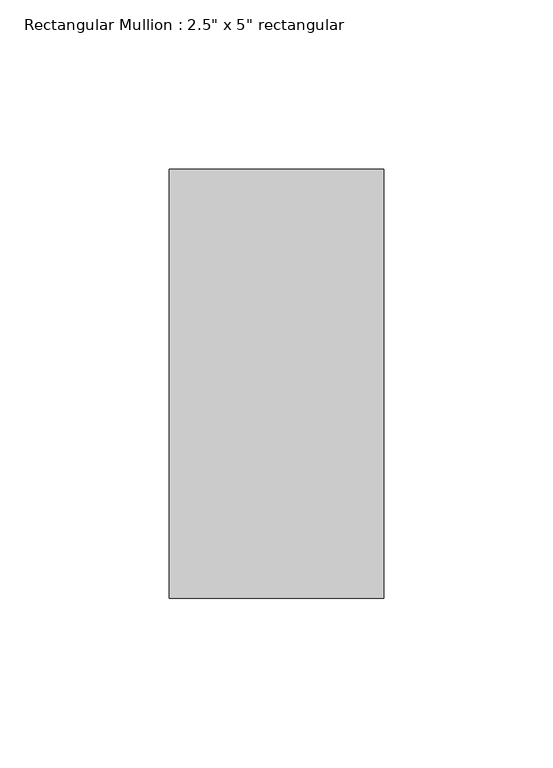
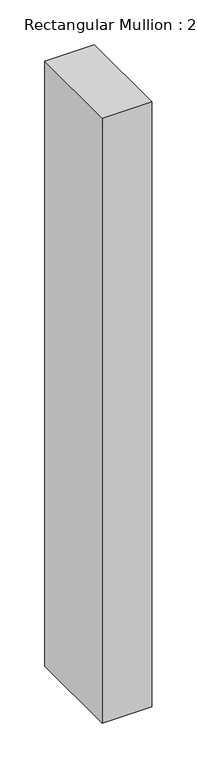
"""IFC4 building model written with IfcOpenShell, lengths in millimetres: member geometry."""

from ifc_helpers import new_model, si_unit, frame, origin, place, context, project, spatial, polyline, outline, extrude, source, transform, mapped, element, save


def member_8ac64e86(model_context):
    return source(origin(), model_context, "Body", "SweptSolid", [
        extrude(outline(polyline([(0.0, 63.5), (0.0, -63.5), (-63.5, -63.5), (-63.5, 63.5), (0.0, 63.5)])), frame((0.0, 0.0, -821.0270145), z_axis=(0.0, 0.0, 1.0), x_axis=(1.0, 0.0, 0.0)), (0.0, 0.0, 1.0), 821.0270145),
    ])


if __name__ == "__main__":
    model = new_model("IFC4")
    model_context = context("Model", 3, world=origin())
    ifc_project = project(units=[si_unit("LENGTHUNIT", "METRE", prefix="MILLI")], contexts=[model_context])
    site = spatial("IfcSite", under=ifc_project)
    building = spatial("IfcBuilding", under=site)
    placement = place(None, origin())
    member_shape = member_8ac64e86(model_context)
    element("IfcMember", 1, ObjectType="Rectangular Mullion : 2.5\" x 5\" rectangular", at=placement, inside=building, context=model_context, shape_type="MappedRepresentation", body=[
        mapped(member_shape, transform((0.0, 0.0, 0.0), x_axis=(1.0, 0.0, 0.0), y_axis=(0.0, 1.0, 0.0), z_axis=(0.0, 0.0, 1.0))),
    ])
    save(model, "model.ifc")

# Revit data of these elements
# Type "Rectangular Mullion : 2.5\" x 5\" rectangular"
#   built-in parameter 1007304 = 0.416667 (stored number, unit not read)
#   built-in parameter 1007301 = 0.104167 (stored number, unit not read)
#   built-in parameter 1007300 = 0.104167 (stored number, unit not read)
# Element 1 (IfcMember, "Rectangular Mullion : 2.5\" x 5\" rectangular")
#   Materials on its faces: "Aluminum"
# Materials
#   "Aluminum": class "Metal", colour RGB 247 247 247, transparency 0, Description = "Aluminum 6061", Cost = 0
